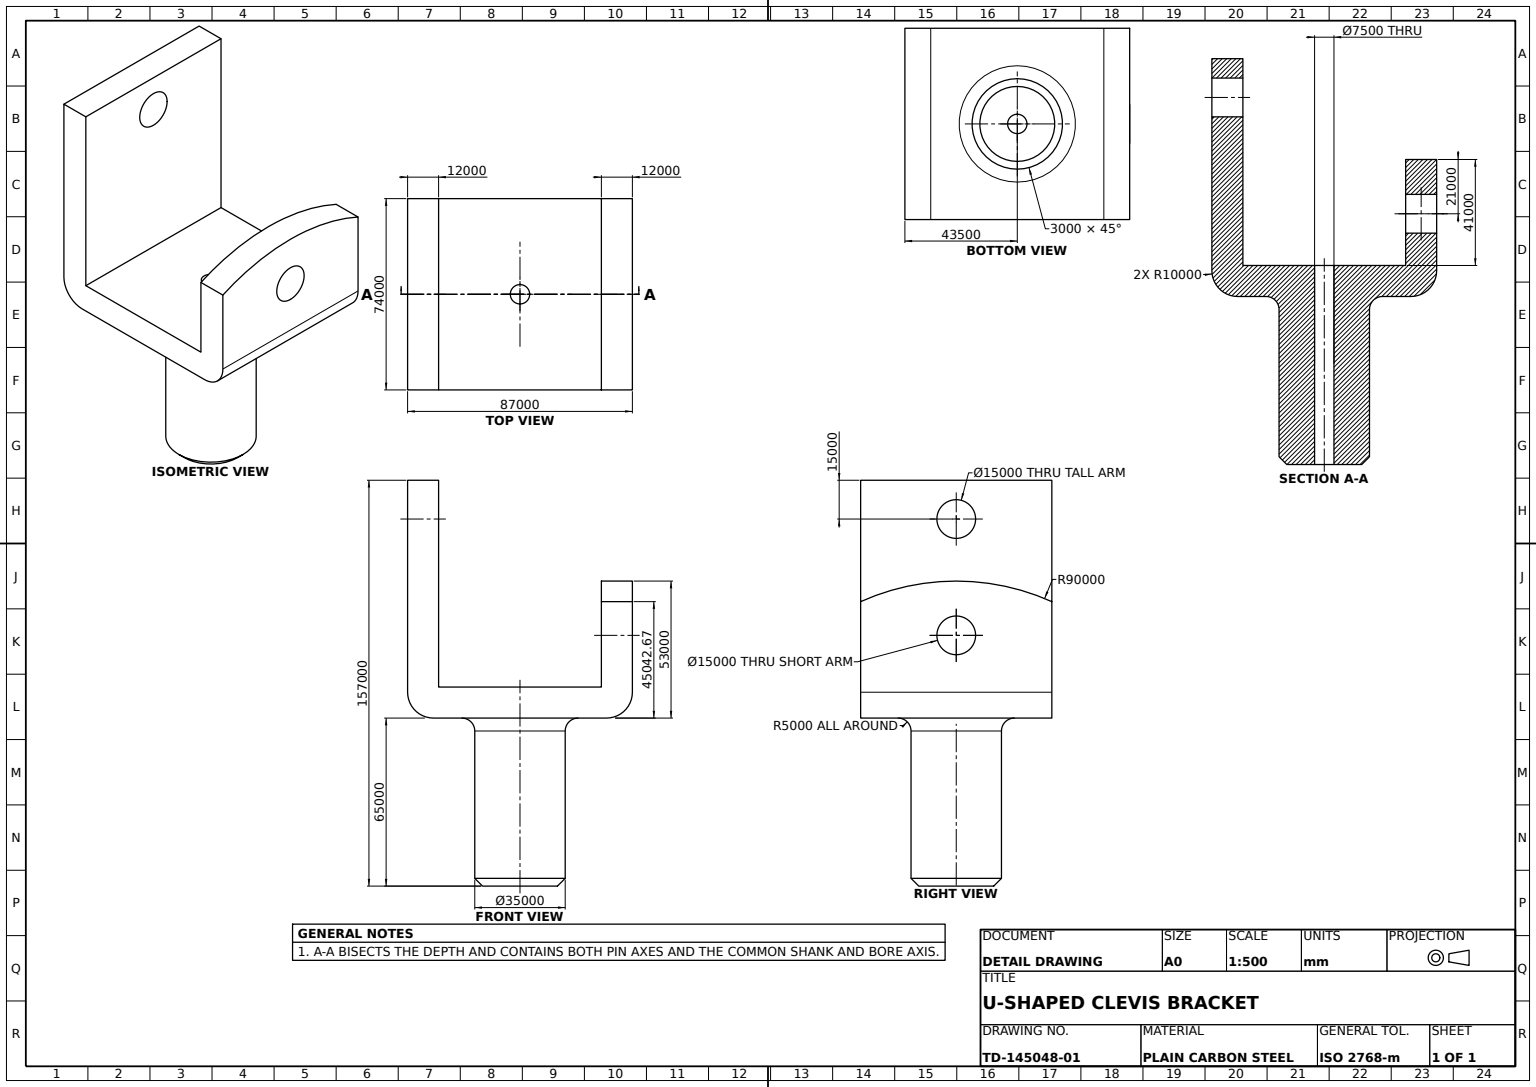
from build123d import *

# Parameters (mm, degrees)
U_BRACKET_BODY_DEPTH                = 37000
CORNER_FILLET_R10_A_R               = 10000
CORNER_FILLET_R10_B_R               = 10000
SHORT_ARM_ARC_TOP_PROFILE_OUTSIDE_W = 103333.894
SHORT_ARM_ARC_TOP_PROFILE_OUTSIDE_H = 121333.894
SHORT_ARM_ARC_TOP_CUT_DEPTH         = 12000
SHORT_ARM_PIN_HOLE_SKETCH_R         = 7500
SHORT_ARM_PIN_HOLE_DEPTH            = 12000
TALL_ARM_PIN_HOLE_SKETCH_R          = 7500
TALL_ARM_PIN_HOLE_DEPTH             = 12000
SHANK_PROFILE_35_R                  = 17500
SHANK_35_DEPTH                      = 65000
SHANK_ROOT_FILLET_R5_R              = 5000
SHANK_END_CHAMFER_3X45_SIZE         = 3000
SHANK_HOLE_SKETCH_7_5_R             = 3750
SHANK_HOLE_7_5_DEPTH                = 167064.61063978


with BuildPart() as part:
    # U Bracket Profile → U Bracket Body (new, symmetric)
    with BuildSketch(Plane.XY):
        Polygon((-31500, 6000), (31500, 6000), (31500, 47000), (43500, 47000), (43500, 6000), (43500, -6000), (-43500, -6000), (-43500, 6000), (-43500, 86000), (-31500, 86000), align=None)
    extrude(amount=U_BRACKET_BODY_DEPTH, both=True)

    # Corner Fillet R10 A
    corner_fillet_r10_a_edges = [part.edges().sort_by_distance(p)[0] for p in [
        (43500, -6000, 0),
    ]]
    fillet(corner_fillet_r10_a_edges, radius=CORNER_FILLET_R10_A_R)

    # Corner Fillet R10 B
    corner_fillet_r10_b_edges = [part.edges().sort_by_distance(p)[0] for p in [
        (-43500, -6000, 0),
    ]]
    fillet(corner_fillet_r10_b_edges, radius=CORNER_FILLET_R10_B_R)

    # Short Arm Arc Top Profile outside → Short Arm Arc Top Cut (cut)
    with BuildSketch(Plane(origin=(43500, 0, 0), x_dir=(0, 0, -1), z_dir=(1, 0, 0))):
        with Locations((0, 40000)):
            Rectangle(SHORT_ARM_ARC_TOP_PROFILE_OUTSIDE_W, SHORT_ARM_ARC_TOP_PROFILE_OUTSIDE_H)
        with BuildLine():
            Line((-37000, 39042.671823875), (-37000, 4000))
            Line((-37000, 4000), (-37000, -6000))
            Line((-37000, -6000), (37000, -6000))
            Line((37000, -6000), (37000, 4000))
            Line((37000, 4000), (37000, 39042.671823875))
            ThreePointArc((37000, 39042.671823875), (0, 47000), (-37000, 39042.671823875))
        make_face(mode=Mode.SUBTRACT)
    extrude(amount=-SHORT_ARM_ARC_TOP_CUT_DEPTH, mode=Mode.SUBTRACT)

    # Short Arm Pin Hole Sketch → Short Arm Pin Hole (cut)
    with BuildSketch(Plane(origin=(43500, 0, 0), x_dir=(0, 0, -1), z_dir=(1, 0, 0))):
        with Locations(Location((0, 26000, 0), (0, 0, 90))):
            Circle(SHORT_ARM_PIN_HOLE_SKETCH_R)
    extrude(amount=-SHORT_ARM_PIN_HOLE_DEPTH, mode=Mode.SUBTRACT)

    # Tall Arm Pin Hole Sketch → Tall Arm Pin Hole (cut)
    with BuildSketch(Plane.ZY.offset(43500)):
        with Locations((0, 71000)):
            Circle(TALL_ARM_PIN_HOLE_SKETCH_R)
    extrude(amount=-TALL_ARM_PIN_HOLE_DEPTH, mode=Mode.SUBTRACT)

    # Shank Profile Ø35 → Shank Ø35 (add)
    with BuildSketch(Plane.XZ.offset(6000)):
        with Locations(Location((0, 0, 0), (0, 0, 90))):
            Circle(SHANK_PROFILE_35_R)
    extrude(amount=SHANK_35_DEPTH)

    # Shank Root Fillet R5
    shank_root_fillet_r5_edges = [part.edges().sort_by_distance(p)[0] for p in [
        (0, -6000, -17500),
    ]]
    fillet(shank_root_fillet_r5_edges, radius=SHANK_ROOT_FILLET_R5_R)

    # Shank End Chamfer 3x45
    shank_end_chamfer_3x45_edges = [part.edges().sort_by_distance(p)[0] for p in [
        (0, -71000, -17500),
    ]]
    chamfer(shank_end_chamfer_3x45_edges, length=SHANK_END_CHAMFER_3X45_SIZE)

    # Shank Hole Sketch Ø7.5 → Shank Hole Ø7.5 (cut, through all)
    with BuildSketch(Plane.XZ.offset(71000)):
        with Locations(Location((0, 0, 0), (0, 0, 270))):
            Circle(SHANK_HOLE_SKETCH_7_5_R)
    extrude(amount=-SHANK_HOLE_7_5_DEPTH, mode=Mode.SUBTRACT)


solid = part.part
